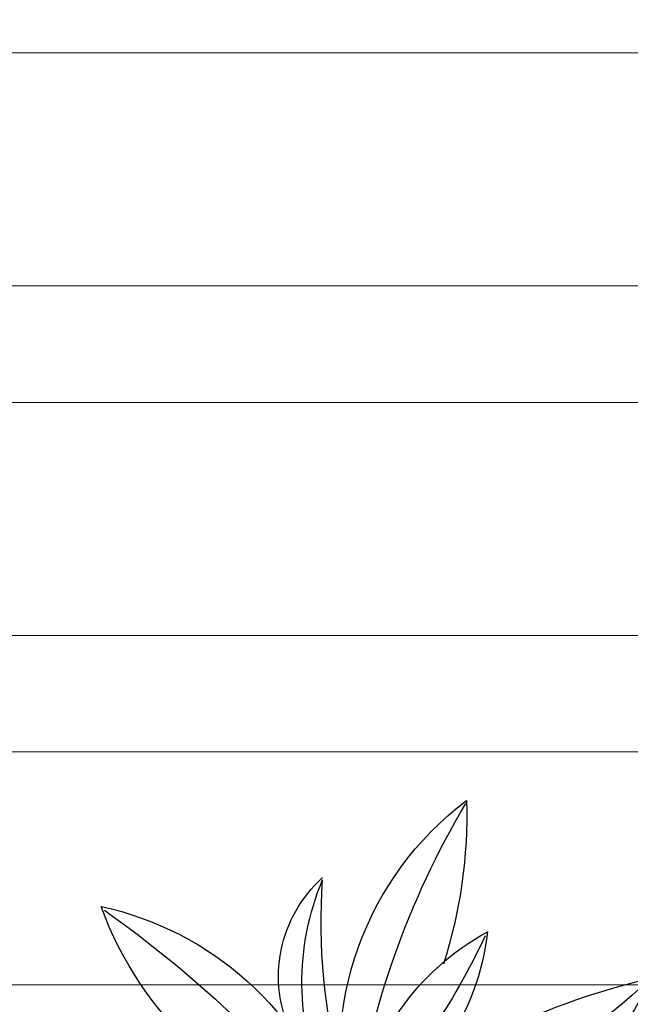
# Model space of a CAD drawing. Units: inches. Extents: x 351 to 1738, y -265 to 286.
# Tile 16 of 38: x 1176 to 1209, y -175 to -122. Entities that reach past the tile are written whole.
import ezdxf

# ---------------------------------------------------------------- set-up
doc = ezdxf.new("R2010")
doc.units = ezdxf.units.IN
doc.header["$MEASUREMENT"] = 0
doc.layers.add('A-ANNO-DIMS', color=2, linetype='Continuous', lineweight=18)
doc.layers.add('A-FLOR-PATT', color=9, linetype='Continuous', lineweight=9)
for name, color, linetype in [('CAY', 94, 'Continuous'), ('CHITIET', 144, 'Continuous'), ('netmanh', 9, 'Continuous'), ('VATDUNG', 9, 'Continuous')]:
    doc.layers.add(name, color=color, linetype=linetype)
doc.styles.get("Standard").update_dxf_attribs({"font": 'arial.ttf'})
doc.dimstyles.get("Standard").update_dxf_attribs({"dimtxt": 8, "dimasz": 5, "dimexe": 0.18, "dimexo": 0.0625, "dimgap": 0.09, "dimtad": 1, "dimtoh": 1, "dimzin": 0, "dimdsep": 46, "dimlunit": 4, "dimtxsty": 'Standard', "dimcen": 0, "dimclre": 256, "dimadec": 0, "dimazin": 0, "dimtfac": 1, "dimtofl": 0, "dimtmove": 0, "dimatfit": 3, "dimfxl": 1, "dimtolj": 1, "dimtzin": 0, "dimlwe": -1, "dimarcsym": 0})

# ---------------------------------------------------------------- blocks, each defined once
blk = doc.blocks.new('A$C5431134F')
at = {"layer": 'VATDUNG'}
for centre, radius, start, end in [((2160.8, 1662), 1245, 150.2411, 205.809), ((5177, 1582.5), 4150.3, 170.24, 186.1148), ((-65.9, 1738.8), 1267.2, 354.3326, 25.2804), ((193.1, 3473.3), 2507.8, 289.6318, 316.9416), ((2357.8, 162.2), 1629.1, 101.2486, 143.9899), ((1000.7, 2213.1), 1133.8, 274.4073, 336.4431), ((1532.8, 1250.1), 499, 101.4267, 190.9877), ((1828.1, 1082.8), 773.2, 121.9055, 175.1859), ((3715.1, 660.2), 2523.5, 154.6853, 162.4501), ((-246.7, 51.1), 1647.5, 39.15, 81.389), ((1000.7, 2213.1), 1133.8, 208.0484, 264.6491), ((1859.5, 3770.4), 2797.6, 228.5745, 252.3842), ((1101.5, 1552.5), 361.2, 169.1166, 218.9556), ((667.9, 1279.8), 349.9, 42.8374, 76.9786), ((-929.9, 388.9), 2082.1, 20.5138, 36.0242), ((1386.4, 1856.4), 738.5, 261.6389, 315.6255), ((-169.9, 6392.7), 5465.7, 286.3355, 292.415), ((1571.2, 1428.8), 356.3, 257.3557, 344.3532), ((624.5, 223.6), 940.4, 92.4374, 115.2956), ((-65.9, 1738.8), 1267.2, 330.7697, 331.9367), ((1294.4, -49.6), 1206.1, 104.1284, 160.1468), ((-2233.8, 3749.8), 4146.2, 305.4464, 320.7382), ((2052.7, 864.5), 1083.3, 166.3603, 232.9474), ((1250.8, 281.5), 836.9, 19.4342, 107.4357), ((625, 349.3), 851.8, 6.5073, 62.3609), ((-70, 1420), 1084.7, 282.2423, 341.7321), ((546.4, 1826.6), 819.5, 246.7315, 287.3971), ((248.9, 8461.8), 7388, 269.91003, 274.50199), ((3885.3, 1488.7), 2894, 188.0959, 210.7226), ((1889.6, 1210.8), 871.9, 188.5552, 241.3289), ((-527.8, -458.7), 2192.5, 24.7599, 44.6473), ((2594.9, 3037.7), 2500, 231.5416, 257.1764), ((754.1, -691.9), 1814.1, 46.1483, 80.3711), ((1738.9, 617.5), 897.6, 155.9893, 202.84), ((2946.5, 414), 2039.9, 165.0604, 184.0737), ((1214.1, 597.8), 452.1, 154.5276, 228.0163), ((-246.7, 51.1), 1647.5, 358.2222, 17.8583)]:
    blk.add_arc(centre, radius, start, end, dxfattribs=at)
blk = doc.blocks.new('A$C5A8625A6')
at = {"layer": 'CHITIET', "ltscale": 50, "xscale": -0.49, "yscale": 0.49, "zscale": 0.49, "rotation": 180}
blk.add_blockref('A$C5431134F', (0, 1120.2), dxfattribs=at)
blk = doc.blocks.new('A$C18571848')
at = {"layer": 'netmanh', "xscale": 0.5393606399999998, "yscale": 0.5393606399999998, "zscale": 0.5393606399999998}
blk.add_blockref('A$C5A8625A6', (0, 0), dxfattribs=at)
blk = doc.blocks.new('*D36')
at = {"layer": 'A-ANNO-DIMS', "transparency": 16777216}
for p, q in [((1073.569, -199.341), (1073.569, -204.202)), ((1105.198, -199.341), (1105.198, -204.202))]:
    blk.add_line(p, q, dxfattribs=at)
at = {"layer": 'A-ANNO-DIMS', "color": 0, "lineweight": -2, "transparency": 16777216}
for p, q in [((1078.569, -204.022), (1100.198, -204.022)), ((1105.198, -204.022), (1227.071, -204.022))]:
    blk.add_line(p, q, dxfattribs=at)
at = {"layer": 'A-ANNO-DIMS', "color": 0, "transparency": 16777216}
for points in [[(1078.569, -203.189), (1078.569, -204.856), (1073.569, -204.022)], [(1100.198, -203.189), (1100.198, -204.856), (1105.198, -204.022)]]:
    blk.add_solid(points, dxfattribs=at)
at = {"layer": 'Defpoints', "color": 0, "transparency": 16777216}
for p in [(1073.569, -199.278), (1105.198, -199.278), (1105.198, -204.022)]:
    blk.add_point(p, dxfattribs=at)
at = {"layer": 'A-ANNO-DIMS', "color": 0, "transparency": 16777216, "insert": (1168.634, -199.796), "char_height": 8, "attachment_point": 5}
blk.add_mtext('\\A1;PLANT A 2\'-7 1/2" TYP.', dxfattribs=at)

msp = doc.modelspace()

# ---------------------------------------------------------------- hatches: boundary and pattern name
at = {"layer": 'A-FLOR-PATT', "transparency": 33554559}
h = msp.add_hatch(dxfattribs=at)
h.set_pattern_fill('ANSI37', color=256, scale=200, angle=135)
h.set_pattern_definition([(180, (1112.704, -164.037), (-2e-15, -25), []), (270, (1112.704, -164.037), (25, -5e-15), [])])
h.paths.add_polyline_path([(1380.064, 73.463), (1380.132, 148.463), (1338.064, 148.463), (1290.704, 148.463), (1290.704, 88.463), (1248.704, 88.463), (1248.704, -2.009), (1244.704, -2.009), (1244.704, 142.457), (1160.704, 142.457), (1160.704, 158.963), (1160.704, 170.137), (1160.704, 206.137), (1160.704, 228.963), (1112.704, 228.963), (1112.704, 209.963), (1112.704, 168.963), (1124.704, 168.963), (1124.704, 162.963), (1112.704, 162.963), (1112.704, 64.463), (1112.704, 60.463), (1112.704, 0.463), (1112.704, -48.026), (1146.804, -47.981), (1146.804, -35.691), (1207.804, -35.691), (1207.804, -47.902), (1236.542, -47.864), (1236.544, -50.009), (1248.5, -50.009), (1248.506, -102.915), (1248.512, -150.915), (1248.514, -164.037), (1248.549, -164.037), (1273.017, -164.037), (1273.017, -128.799), (1355.24, -128.799), (1355.24, -164.037), (1384.204, -164.037), (1384.204, -57.037), (1380.064, -57.037), (1380.064, -48.037), (1392.064, -48.037), (1392.064, -53.037), (1406.549, -53.037), (1406.549, -57.037), (1401.204, -57.037), (1401.204, -147.037), (1468.204, -147.037), (1468.204, -138.5), (1472.204, -138.5), (1472.204, -102.5), (1468.204, -102.5), (1468.204, -57.037), (1442.549, -57.037), (1442.549, -53.037), (1463.049, -53.037), (1463.049, -40.747), (1524.049, -40.747), (1524.049, -48.037), (1536.064, -48.037), (1536.064, -53.037), (1557.704, -53.037), (1557.704, 204.963), (1384.204, 204.963), (1384.204, 73.463), (1392.064, 73.463), (1392.064, 64.463), (1384.204, 64.463), (1384.204, -3.5), (1380.204, -3.537), (1380.204, 64.463), (1380.064, 64.463)])
h.paths.add_polyline_path([(1510.714, 86.458, -0.103984), (1511.661, 85.595, 0.470438), (1510.158, 87.614, 0.0961)], flags=16)
h.paths.add_polyline_path([(1510.443, 100.266, 0.009798), (1504.693, 100.48, 0.02879), (1504.6, 99.767, -0.165331), (1505.519, 96.135, -0.143601)], flags=16)
h.paths.add_polyline_path([(1487.201, 85.595, -0.103984), (1488.148, 86.458, 0.0961), (1488.704, 87.614, 0.470438)], flags=0)
h.paths.add_polyline_path([(1495.052, 100.43), (1494.178, 100.43, -0.026463), (1494.262, 99.774, -0.144219)], flags=16)
h.paths.add_polyline_path([(1444.485, 86.458, -0.103984), (1445.433, 85.595, 0.470438), (1443.93, 87.614, 0.0961)], flags=16)
h.paths.add_polyline_path([(1420.972, 85.595, -0.103984), (1421.92, 86.458, 0.0961), (1422.475, 87.614, 0.470438)], flags=16)
h.paths.add_polyline_path([(1428.632, 100.335, 0.001054), (1427.971, 100.309, -0.021524), (1428.033, 99.774, -0.114301)], flags=16)
h.paths.add_polyline_path([(1419.906, 143.708, 0.024979), (1420.222, 157.526), (1421.573, 159.101), (1421.573, 175.369), (1391.393, 175.369), (1391.393, 200.519), (1542.294, 200.519), (1542.294, 175.369), (1512.028, 175.369, 0.019865), (1511.521, 153.838, 0.025134), (1512.758, 118.323, 0.020553), (1512.942, 115.253), (1419.834, 115.253, -0.000414), (1419.843, 124.798), (1413.059, 124.798), (1413.059, 84.437, -0.061853), (1415.831, 80.45, -0.093077), (1420.972, 85.595, -0.267537), (1422.371, 84.732, 0.08511), (1424.052, 84.616, -0.885393), (1424.033, 84.851, -1.125815), (1424.073, 84.366, -0.087987), (1422.371, 84.732, -0.267537), (1422.326, 83.089, -0.370542), (1420.972, 85.595, 0.093077), (1415.831, 80.45, -0.087414), (1417.914, 73.937), (1418.941, 73.937, 0.02725), (1418.913, 76.906, -0.115703), (1421.051, 73.937), (1445.354, 73.937, -0.115703), (1447.492, 76.906, 0.02725), (1447.464, 73.937), (1448.491, 73.937, -0.087414), (1450.574, 80.45, 0.093077), (1445.433, 85.595, -0.370542), (1444.079, 83.089, -0.267537), (1444.034, 84.732, -0.087987), (1442.332, 84.366, -1.125815), (1442.372, 84.851, -2.032736), (1442.364, 84.368, 0.086378), (1444.034, 84.732, -0.267537), (1445.433, 85.595, -0.093077), (1450.574, 80.45, -0.257732), (1466.483, 90.927, -0.47867), (1468.832, 91.907, -0.47867), (1471.18, 90.927, -0.26264), (1483.053, 81.78, -0.071866), (1487.201, 85.595, -0.267537), (1488.6, 84.732, 0.08511), (1490.28, 84.616, -0.885393), (1490.262, 84.851, -1.125815), (1490.301, 84.366, -0.087987), (1488.6, 84.732, -0.267537), (1488.554, 83.089, -0.370542), (1487.201, 85.595, 0.071866), (1483.053, 81.78, -0.132065), (1484.143, 73.937), (1485.169, 73.937, 0.02725), (1485.142, 76.906, -0.115703), (1487.28, 73.937), (1511.582, 73.937, -0.115703), (1513.72, 76.906, 0.02725), (1513.693, 73.937), (1514.719, 73.937, -0.087414), (1516.802, 80.45, 0.093077), (1511.661, 85.595, -0.370542), (1510.308, 83.089, -0.267537), (1510.262, 84.732, -0.087987), (1508.561, 84.366, -1.125815), (1508.601, 84.851, -2.032736), (1508.592, 84.368, 0.086378), (1510.262, 84.732, -0.267537), (1511.661, 85.595, -0.093077), (1516.802, 80.45, -0.061853), (1519.575, 84.437), (1519.575, 73.937), (1413.059, 73.937), (1413.059, 124.798), (1419.843, 124.798, -0.000821)], flags=16)
h.paths.add_polyline_path([(1220.149, 54.133, -0.103984), (1220.869, 53.476, 0.470438), (1219.727, 55.011, 0.0961)], flags=16)
h.paths.add_polyline_path([(1219.944, 64.626, 0.009798), (1215.574, 64.789, 0.02879), (1215.503, 64.247, -0.165331), (1216.201, 61.487, -0.143601)], flags=16)
h.paths.add_polyline_path([(1209.779, 64.449, 0.097446), (1209.339, 64.751), (1208.247, 64.751, 0.12739), (1207.7, 64.326, 0.171586), (1206.95, 61.475, -0.158854), (1207.636, 59.45, 0.015898), (1207.795, 59.218, 0.061546), (1208.598, 59.616, 0.175416), (1208.638, 60.099, -0.284779), (1209.348, 62.472, 0.326216)], flags=16)
h.paths.add_polyline_path([(1169.818, 54.133, -0.103984), (1170.538, 53.476, 0.470438), (1169.396, 55.011, 0.0961)], flags=16)
h.paths.add_polyline_path([(1159.017, 62.472, 0.284764), (1158.307, 60.099, -0.175433), (1158.267, 59.616, 0.39293), (1159.448, 64.449, -0.32623)], flags=16)
h.paths.add_polyline_path([(1156.342, 58.239, -0.178321), (1154.011, 55.31, -0.174736), (1154.722, 55.233, -0.200802), (1156.27, 56.086, 0.12699), (1157.283, 58.991, -0.091205)], flags=16)
h.paths.add_polyline_path([(1156.624, 61.413, 0.157275), (1157.316, 64.247, 0.169622)], flags=16)
h.paths.add_polyline_path([(1152.67, 54.133, -0.0961), (1151.95, 53.476, 0.064076), (1154.465, 54.384, 0.199016)], flags=16)
h.paths.add_polyline_path([(1202.281, 53.476, -0.103984), (1203, 54.133, 0.0961), (1203.423, 55.011, 0.470438)], flags=0)
h.paths.add_polyline_path([(1151.139, 97.64, 0.024979), (1151.379, 108.141), (1152.406, 109.338), (1152.406, 121.701), (1129.47, 121.701), (1129.47, 140.814), (1244.149, 140.814), (1244.149, 121.701), (1221.148, 121.701, 0.019865), (1220.763, 105.338, 0.025134), (1221.703, 78.349, 0.020553), (1221.843, 76.016), (1151.078, 76.016, -0.128743), (1148.786, 65.037, 0.539352), (1150.327, 64.171, -0.027594), (1163.481, 64.751, 0.097695), (1163.04, 64.449, 0.326216), (1163.471, 62.472, -0.284777), (1164.181, 60.099, -0.194757), (1165.846, 61.443, -0.155402), (1165.172, 64.247, -0.166022), (1165.869, 61.475, -0.177014), (1167.852, 62.77, -0.448203), (1169.974, 60.807, -0.393499), (1167.679, 57.86, -0.895548), (1168.438, 54.524, -0.355767), (1166.218, 56.086, -0.066024), (1165.505, 57.539), (1165.251, 56.243, -0.371732), (1164.02, 59.758, -0.373614), (1163.04, 64.449, -0.097695), (1163.481, 64.751, 0.021354), (1153.294, 64.429, -0.134183), (1156.695, 61.368, 0.186873), (1154.636, 62.77, 0.448203), (1152.514, 60.807, 0.403726), (1154.905, 57.846, 0.711219), (1153.334, 55, 0.53154), (1151.95, 53.476, -0.267537), (1153.013, 52.821, 0.08511), (1154.29, 52.732, -0.885393), (1154.276, 52.911, -1.125815), (1154.306, 52.543, -0.087987), (1153.013, 52.821, -0.267537), (1152.978, 51.572, -0.370542), (1151.95, 53.476, 0.093077), (1148.043, 49.566, -0.087414), (1149.626, 44.617), (1150.406, 44.617, 0.02725), (1150.385, 46.873, -0.115703), (1152.01, 44.617), (1170.478, 44.617, -0.115703), (1172.103, 46.873, 0.02725), (1172.082, 44.617), (1172.862, 44.617, -0.087414), (1174.445, 49.566, 0.093077), (1170.538, 53.476, -0.370542), (1169.51, 51.572, -0.267537), (1169.475, 52.821, -0.087987), (1168.182, 52.543, -1.125815), (1168.212, 52.911, -2.032736), (1168.206, 52.544, 0.086378), (1169.475, 52.821, -0.267537), (1170.538, 53.476, -0.093077), (1174.445, 49.566, -0.257732), (1186.536, 57.528, -0.47867), (1188.321, 58.273, -0.47867), (1190.106, 57.528, -0.26264), (1199.128, 50.577, -0.071866), (1202.281, 53.476, -0.267537), (1203.344, 52.821, 0.08511), (1204.621, 52.732, -0.885393), (1204.607, 52.911, -1.125815), (1204.637, 52.543, -0.087987), (1203.344, 52.821, -0.267537), (1203.309, 51.572, -0.370542), (1202.281, 53.476, 0.071866), (1199.128, 50.577, -0.132065), (1199.957, 44.617), (1200.737, 44.617, 0.02725), (1200.716, 46.873, -0.115703), (1202.341, 44.617), (1220.809, 44.617, -0.115703), (1222.434, 46.873, 0.02725), (1222.413, 44.617), (1223.193, 44.617, -0.087414), (1224.776, 49.566, 0.093077), (1220.869, 53.476, -0.370542), (1219.841, 51.572, -0.267537), (1219.806, 52.821, -0.087987), (1218.513, 52.543, -1.125815), (1218.543, 52.911, -2.032736), (1218.537, 52.544, 0.086378), (1219.806, 52.821, -0.267537), (1220.869, 53.476, -0.093077), (1224.776, 49.566, -0.061853), (1226.883, 52.597), (1226.883, 44.617), (1145.936, 44.617), (1145.936, 83.269), (1151.091, 83.269, -0.000821)], flags=16)
h.paths.add_polyline_path([(1218.01, 57.86, -0.895548), (1218.769, 54.524, -0.355767), (1216.549, 56.086, -0.066024), (1215.836, 57.539), (1215.582, 56.243, -0.371732), (1214.351, 59.758, -0.373614), (1213.371, 64.449, 0.326216), (1213.802, 62.472, -0.284777), (1214.512, 60.099, -0.194757), (1216.177, 61.443, -0.179991), (1218.183, 62.77, -0.448203), (1220.305, 60.807, -0.393499)], flags=16)
h.paths.add_polyline_path([(1424.735, 91.363, -0.393499), (1421.715, 95.241, -0.448203), (1424.507, 97.824, -0.179991), (1427.147, 96.077, -0.194757), (1429.338, 94.309, -0.284777), (1430.272, 97.432, 0.326216), (1430.839, 100.034, -0.373614), (1429.55, 93.861, -0.371732), (1427.929, 89.235), (1427.596, 90.941, -0.066024), (1426.657, 89.029, -0.355767), (1423.736, 86.973, -0.895548)], flags=16)
h.paths.add_polyline_path([(1238.033, 131.257, -1), (1227.329, 131.257, -1)], flags=0)
h.paths.add_polyline_path([(1235.357, 131.257, -1), (1230.005, 131.257, -1)], flags=0)
h.paths.add_polyline_path([(1214.039, 54.243, 0.154382), (1214.38, 53.992, 0.358955), (1213.613, 54.016, 0.603948), (1214.379, 53.657, 0.371319), (1213.968, 52.872, 0.187994), (1214.312, 52.809, -0.592455), (1213.953, 52.967, -0.294279), (1214.083, 53.691, -1.300187), (1213.881, 54.134, -0.283762), (1214.469, 53.896, 1.15094)], flags=16)
h.paths.add_polyline_path([(1212.091, 56.286, -0.408434), (1211.337, 56.445, -0.036259), (1211.098, 56.848, -0.236098), (1211.59, 56.63, 0.035345), (1211.835, 56.543, -0.475241), (1212.091, 56.286, -0.475241), (1212.438, 56.182, 0.035345), (1212.631, 56.007, -0.236098), (1213.056, 55.676, -0.036259), (1212.588, 55.697, -0.408434)], flags=16)
h.paths.add_polyline_path([(1211.469, 50.297, 0.296043), (1210.47, 50.527, 0.310883), (1211.931, 50.148, 0.021255)], flags=16)
h.paths.add_polyline_path([(1213.739, 51.818, -0.036259), (1213.271, 51.838, -0.408434), (1212.774, 52.427, -0.094786), (1212.293, 50.703, 1.150474), (1212.911, 50.232, 0.166288), (1213.265, 50.68, -0.025254), (1212.603, 50.13, 1.087932), (1212.471, 49.407, 0.166288), (1213.02, 49.251, -0.016128), (1212.567, 49.563, -0.286859), (1212.217, 49.638, 0.022156), (1212.046, 50.055, -0.64613), (1212.185, 50.498, 0.088412), (1212.732, 52.077, -1.186037), (1213.121, 52.323, 0.035345), (1213.314, 52.148, -0.236098)], flags=16)
h.paths.add_polyline_path([(1212.094, 50.342, -0.048524), (1211.54, 49.605, -1.103834), (1211.397, 48.738, -0.785515), (1211.683, 48.254, -0.392043), (1210.948, 48.525, -0.392819), (1210.561, 47.995, -0.592455), (1210.201, 48.153, -0.294279), (1210.331, 48.877, -0.704172), (1210.316, 49.592, -0.679344), (1210.729, 50.112, 0.563676)], flags=16)
h.paths.add_polyline_path([(1211.274, 49.829, -0.139826), (1210.745, 49.859, -0.217879), (1210.948, 49.509, -0.498572)], flags=0)
h.paths.add_polyline_path([(1433.426, 81.49, -0.181571), (1434.245, 81.788, -0.008067), (1433.726, 82.205, 0.045578), (1432.755, 81.242, 0.179011)], flags=16)
h.paths.add_polyline_path([(1434.146, 81.009, -0.132442), (1433.645, 80.771, 0.259089), (1433.234, 80.471, -0.180211), (1433.392, 80.805, -0.16994), (1432.758, 81.109, 0.032652), (1433.273, 80.474, -0.493363), (1434.046, 80.146, -0.390497)], flags=16)
h.paths.add_polyline_path([(1434.83, 80.047, -0.947538), (1435.294, 79.576, -0.299128), (1434.625, 79.404, -0.270439), (1435.01, 78.591, -0.592455), (1434.537, 78.382, -0.392819), (1434.027, 79.08, -0.392043), (1433.06, 78.723, -0.352042), (1433.003, 79.197, -0.197216), (1433.75, 79.734, -0.71364), (1434.447, 79.939, -0.21479), (1434.819, 80.475, 0.408833), (1435.075, 80.803, -0.226152)], flags=16)
h.paths.add_polyline_path([(1432.67, 81.217, -0.454218), (1431.897, 79.923, -0.414411), (1431.301, 80.035, 0.016129), (1431.897, 80.445, 0.27957), (1432.073, 80.871, -0.289504), (1431.103, 81.321, -0.414411), (1430.978, 81.915, 0.01613), (1431.586, 81.521, 0.341293), (1432.125, 81.583, -0.813186)], flags=16)
h.paths.add_polyline_path([(1429.893, 86.381, -0.947538), (1430.358, 85.91, -0.173106), (1429.984, 85.712, -0.038817), (1431.625, 84.214, -0.0879), (1432.097, 88.549, -0.049768), (1431.254, 88.49, -0.236098), (1431.814, 88.925, 0.035345), (1432.067, 89.155, -0.475241), (1432.524, 89.291, -0.475241), (1432.86, 89.63, 0.035345), (1433.182, 89.744, -0.236098), (1433.83, 90.032, -0.036259), (1433.516, 89.502, -0.408434), (1432.524, 89.291, -0.312424), (1432.106, 88.58, 0.088559), (1431.625, 84.214, -0.408434), (1430.971, 83.439, -0.036259), (1430.355, 83.412, -0.236098), (1430.914, 83.847, 0.035345), (1431.168, 84.078, -0.475241), (1431.625, 84.214, 0.038817), (1429.984, 85.712, -0.321732), (1429.333, 86.048, -0.32743), (1429.883, 86.809, 0.408833), (1430.138, 87.138, -0.226152)], flags=16)
h.paths.add_polyline_path([(1211.206, 58.616, -0.999784), (1211.336, 59.323, -0.614994)], flags=16)
h.paths.add_polyline_path([(1210.288, 49.429, 0.154382), (1210.629, 49.178, 0.358955), (1209.861, 49.202, 0.603948), (1210.627, 48.843, -0.534825), (1210.806, 49.295, 0.748346)], flags=16)
h.paths.add_polyline_path([(1209.589, 51.828, -0.008791), (1209.775, 51.753, 0.112231), (1209.466, 52.019, 1.418851), (1209.014, 51.708, -0.458726), (1208.651, 51.073, -0.592455), (1208.291, 51.232, -0.294279), (1208.421, 51.955, -1.300187), (1208.219, 52.398, -0.226005), (1208.719, 52.257, -0.475519), (1209.158, 52.369, -1.455499), (1209.603, 52.664, 0.421305), (1209.191, 52.262, -0.591212), (1208.979, 51.796, 0.497399), (1209.773, 51.333, 0.649312)], flags=16)
h.paths.add_polyline_path([(1208.029, 52.041, 0.544667), (1208.832, 52.045, 0.220132)], flags=0)
h.paths.add_polyline_path([(1210.438, 51.425, -0.2042), (1210.277, 52.018, 0.270826), (1209.915, 52.897, 0.324115)], flags=0)
h.paths.add_polyline_path([(1209.668, 52.407, -0.60139), (1208.99, 52.221, -0.394916), (1208.248, 52.83, -0.836792), (1208.651, 53.017, -0.338488), (1209.039, 52.571, 0.194138), (1209.191, 52.262, 0.413995), (1209.712, 52.475, 0.51771), (1210.503, 51.416, 0.401922), (1209.493, 50.93, 0.206396), (1209.516, 50.165, -0.319463), (1210.417, 51.418, -0.466635)], flags=16)
h.paths.add_polyline_path([(1206.601, 56.086, -0.355767), (1204.381, 54.524, -0.921198), (1205.236, 57.846, 0.206569), (1207.614, 58.991, -0.12699)], flags=16)
h.paths.add_polyline_path([(1435.487, 82.816, 0.527765), (1436.615, 83.361, 0.50854), (1437.05, 82.433, 0.592455), (1437.524, 82.641, 0.331245), (1436.963, 83.548, 0.387863), (1437.808, 83.626, 0.592954), (1437.618, 84.176, 0.226016), (1436.961, 83.99, 0.318205), (1437.588, 84.854, 0.689374), (1437.05, 84.991, 0.335765), (1436.539, 84.41, -0.156993), (1436.404, 84.065, -0.434611), (1436.961, 83.99, -0.21479), (1437.333, 84.526, 0.408833), (1437.588, 84.854, -0.226152), (1437.343, 84.097, -0.947538), (1437.808, 83.626, -0.299128), (1437.139, 83.455, -0.270439), (1437.524, 82.641, -0.592455), (1437.05, 82.433, -0.392819), (1436.541, 83.13, -0.43966), (1435.475, 82.794, -0.174614), (1435.942, 82.244, -0.206396), (1435.912, 81.237, -0.270826), (1435.125, 82.208, 0.207976), (1434.686, 82.904, -0.196495)], flags=16)
h.paths.add_polyline_path([(1435.386, 84.832, 0.270811), (1434.91, 83.676, -0.204217), (1434.699, 82.895, 0.324115)], flags=0)
h.paths.add_polyline_path([(1435.68, 84.18, -0.217656), (1435.554, 83.304, -0.176705), (1436.236, 83.778, -0.373036)], flags=0)
h.paths.add_polyline_path([(1435.566, 100.034, 0.326216), (1436.133, 97.432, -0.284777), (1437.067, 94.309, -0.194757), (1439.258, 96.077, -0.155402), (1438.371, 99.767, -0.166022), (1439.289, 96.12, -0.177014), (1441.897, 97.824, -0.448203), (1444.69, 95.241, -0.393499), (1441.67, 91.363, -0.895548), (1442.669, 86.973, -0.355767), (1439.748, 89.029, -0.066024), (1438.809, 90.941), (1438.476, 89.235, -0.371732), (1436.855, 93.861, -0.373614)], flags=16)
h.paths.add_polyline_path([(1191.252, 49.507, -0.274022), (1190.658, 48.409, 0.267537), (1191.311, 47.344, 0.370542)], flags=0)
h.paths.add_polyline_path([(1190.301, 49.717, 0.199016), (1188.619, 49.04, 0.064076), (1191.252, 49.507, -0.0961)], flags=0)
h.paths.add_polyline_path([(1189.518, 47.857, 1.125815), (1189.676, 47.523, 2.044605)], flags=0)
h.paths.add_polyline_path([(1464.974, 80.372, 0.274022), (1465.756, 78.927, -0.083013)], flags=0)
h.paths.add_polyline_path([(1464.974, 80.372, 0.370542), (1464.897, 77.525, 0.576324)], flags=0)
h.paths.add_polyline_path([(1464.974, 80.372, -0.470438), (1467.284, 81.372, -0.0961), (1466.226, 80.648, -0.199016), (1468.439, 79.757, -0.064076)], flags=0)
h.paths.add_polyline_path([(1189.511, 56.43, -0.259467), (1188.321, 56.391, -0.259467), (1187.13, 56.43, 0.08511), (1188.193, 55.716, -0.885393), (1188.27, 55.878, -1.196013), (1188.355, 55.442, 0.101459)], flags=0)
h.paths.add_polyline_path([(1188.321, 57.596, 0.078072), (1187.678, 57.24, 0.01555), (1188.321, 57.136, 0.01555), (1188.964, 57.24, 0.078072)], flags=0)
h.paths.add_polyline_path([(1190.164, 55.365, -0.576324), (1190.106, 57.528, -0.198294), (1188.321, 58.319, -0.198294), (1186.536, 57.528, -0.576324), (1186.477, 55.365, -0.370542), (1186.536, 57.528, 0.198294), (1188.321, 58.319, 0.198294), (1190.106, 57.528, -0.370542)], flags=0)
h.paths.add_polyline_path([(1188.372, 55.878, 1.125814), (1188.529, 55.544, 2.044605)], flags=0)
h.paths.add_polyline_path([(1186.341, 49.717, -0.0961), (1185.389, 49.507, 0.064076), (1188.022, 49.04, 0.199016)], flags=0)
h.paths.add_polyline_path([(1185.389, 49.507, -0.267537), (1185.984, 48.409, 0.08511), (1187.046, 47.695, -0.885393), (1187.123, 47.857, -1.125815), (1186.966, 47.523, -0.087987), (1185.984, 48.409, -0.267537), (1185.331, 47.344, -0.370542)], flags=0)
h.paths.add_polyline_path([(1399.441, 187.944, -1), (1413.525, 187.944, -1)], flags=0)
h.paths.add_polyline_path([(1402.962, 187.944, -1), (1410.004, 187.944, -1)], flags=0)
h.paths.add_polyline_path([(1357.663, -72.245), (1377.272, -72.245), (1377.272, -91.854), (1357.663, -91.854)], flags=16)
h.paths.add_polyline_path([(1467.256, 78.201, -1.125815), (1467.049, 77.761, -2.044605)], flags=0)
h.paths.add_polyline_path([(1468.822, 88.714, 0.941125), (1469.106, 88.316, 1.137152), (1468.765, 88.755, 0.890986), (1468.99, 88.245, 0.094828), (1470.398, 89.481, -0.267537), (1471.18, 90.927, -0.028123), (1469.678, 90.547, -0.028774), (1469.948, 90.311, -0.020327), (1468.832, 90.41, -0.020327), (1467.716, 90.311, -0.028774), (1467.986, 90.547, -0.028123), (1466.483, 90.927, -0.267537), (1467.265, 89.481, 0.08511), (1468.663, 88.542, -1.202316)], flags=0)
h.paths.add_polyline_path([(1178.25, 124.523, -0.119929), (1165.65, 124.145, -0.107349), (1159.133, 124.446, -0.102891), (1159.132, 130.465, -0.074897), (1158.993, 137.956, 0.002027), (1167.844, 137.479, -0.07553), (1180.337, 137.666, -0.075861), (1186.502, 137.688, -0.14099), (1186.272, 130.046, -0.095481), (1186.729, 124.748, -0.10603)], flags=0)
h.paths.add_polyline_path([(1469.225, 79.757, -0.199016), (1471.437, 80.648, -0.0961), (1470.379, 81.372, -0.470438), (1472.689, 80.372, -0.370542), (1472.766, 77.525, -0.267537), (1471.907, 78.927, -0.087986), (1470.615, 77.761, -1.125849), (1470.408, 78.201, -2.032736), (1470.642, 77.778, 0.086378), (1471.907, 78.927, -0.267537), (1472.689, 80.372, -0.064076)], flags=0)
h.paths.add_polyline_path([(1430.423, 186.902, -0.074897), (1430.24, 196.758, 0.002027), (1441.887, 196.131, -0.07553), (1458.326, 196.377, -0.075861), (1466.438, 196.406, -0.14099), (1466.136, 186.35, -0.095481), (1466.737, 179.378, -0.10603), (1455.58, 179.082, -0.119929), (1439, 178.585, -0.107349), (1430.425, 178.981, -0.102891)], flags=0)
h.paths.add_polyline_path([(1162.258, 49.939, 0.335765), (1161.87, 49.497, -0.156994), (1161.767, 49.235, -0.434611), (1162.19, 49.178, -0.21479), (1162.473, 49.585, 1.529195)], flags=16)
h.paths.add_polyline_path([(1161.683, 49.021, 0.581518), (1161.268, 49.583, 0.592761)], flags=16)
h.paths.add_polyline_path([(1162.602, 48.058, 0.371319), (1162.192, 48.843, 0.434533), (1162.88, 48.962, 0.185081), (1162.197, 48.926, 1.121837)], flags=16)
h.paths.add_polyline_path([(1161.443, 48.941, -1.307104), (1161.495, 48.571, -0.217752), (1161.136, 48.254, 0.697303), (1161.871, 49.048, 0.121514)], flags=16)
h.paths.add_polyline_path([(1162.531, 49.429, -0.207084), (1162.05, 49.146, -0.99203)], flags=16)
h.paths.add_polyline_path([(1161.304, 49.578, -0.719667), (1161.513, 50.079, -0.130428), (1160.836, 50.168, 0.039593)], flags=0)
h.paths.add_polyline_path([(1162.036, 50.584, -0.008067), (1161.642, 50.9, 0.029367), (1161.35, 50.297, -0.205788)], flags=16)
h.paths.add_polyline_path([(1162.882, 51.392, -0.124733), (1162.763, 51.828, -0.101191), (1162.399, 51.438, -0.153425)], flags=0)
h.paths.add_polyline_path([(1164.235, 51.85, -0.309107), (1164.513, 51.136, -0.627125), (1163.781, 51.603, -0.685909), (1162.777, 51.219, -0.233285), (1163.303, 50.165, -0.270826), (1162.705, 50.903, 0.2042), (1162.381, 51.425, 0.204182), (1162.542, 52.018, -0.270841), (1162.903, 52.897, -0.127261), (1163.219, 52.529, -1.168681), (1163.781, 52.587, -0.329112), (1164.168, 53.017, -0.836792), (1164.571, 52.83, -0.193341), (1164.391, 52.338, -0.947538), (1164.744, 51.981, -0.299128)], flags=16)
h.paths.add_polyline_path([(1163.598, 51.937, -1.262956), (1163.236, 51.831, 0.012575), (1162.971, 51.721, 0.230657), (1163.151, 52.407, -0.164898), (1163.178, 52.661, -0.44932), (1163.628, 52.262, -0.721477), (1164.154, 52.088, -0.849998)], flags=0)
h.paths.add_polyline_path([(1161.613, 58.616, -0.980413), (1161.525, 59.049, -2.908935)], flags=16)
h.paths.add_polyline_path([(1160.252, 49.166, -0.414411), (1159.799, 49.251, 0.016129), (1160.252, 49.563, 0.27957), (1160.386, 49.887, -0.289504), (1159.649, 50.229, -0.414411), (1159.554, 50.68, 0.01613), (1160.015, 50.381, 0.617885), (1160.526, 50.703, -0.094786), (1160.045, 52.427, -0.140444), (1159.682, 52.042, -0.057856), (1159.3, 51.872, 0.544843), (1160.046, 52.419, -0.088122), (1160.404, 55.721, -0.049768), (1159.763, 55.676, -0.236098), (1160.188, 56.007, 0.035345), (1160.381, 56.182, -0.475241), (1160.728, 56.286, -0.475241), (1160.984, 56.543, 0.035345), (1161.229, 56.63, -0.236098), (1161.721, 56.848, -0.036259), (1161.482, 56.445, -0.408434), (1160.728, 56.286, -0.312424), (1160.411, 55.745, 0.088559), (1160.045, 52.427, 0.107081), (1160.634, 50.498, -0.494798), (1160.839, 50.149, -0.454218)], flags=16)
h.paths.add_polyline_path([(1160.666, 49.808, -2.076528), (1160.828, 50.172, 0.019586)], flags=0)
h.paths.add_polyline_path([(1158.439, 53.992, 0.154382), (1158.78, 54.243, 0.748346), (1158.262, 54.109, -0.338225), (1158.492, 53.839, -0.170816), (1159.124, 53.779, 0.495729), (1158.938, 54.134, 0.226016)], flags=16)
h.paths.add_polyline_path([(1160.045, 52.427, 0.038817), (1158.798, 53.565, -0.119818), (1158.574, 53.586, -0.309107), (1158.851, 52.872, -0.187994), (1158.506, 52.809, 0.592455), (1158.866, 52.967, 0.331245), (1158.44, 53.657, 0.201245), (1158.798, 53.565, -0.034023), (1159.901, 52.578, -0.044253), (1159.698, 52.323, -0.475241)], flags=16)
h.paths.add_polyline_path([(1336.926, -95.392), (1336.926, -117.945), (1291.82, -117.945), (1291.82, -95.392)], flags=16)
h.paths.add_polyline_path([(1357.535, -97.244), (1357.726, -96.697, 0.034844)], flags=16)
h.paths.add_polyline_path([(1376.693, -96.478), (1377.301, -96.5, 0.031497), (1375.907, -96.424), (1357.726, -96.424)], flags=16)
h.paths.add_polyline_path([(1379.403, -119.667, 0.026706), (1380.043, -119.439, -0.015299)], flags=16)
h.paths.add_polyline_path([(1357.726, -120.202), (1357.821, -120.202), (1357.821, -120.201)], flags=16)
h.paths.add_polyline_path([(1354.171, -104.592), (1354.469, -98.672, 0.011138)], flags=16)
h.paths.add_polyline_path([(1355.058, -119.136), (1354.578, -118.539, 0.143164)], flags=16)
h.paths.add_polyline_path([(1378.851, -96.821), (1378.85, -96.82), (1378.85, -96.82, -0.04968), (1380.055, -97.191), (1378.85, -96.82, 0.150054), (1375.135, -97.188), (1375.136, -119.44, -0.00997), (1374.747, -116.649), (1357.726, -116.649, 0.169385), (1357.535, -119.382), (1357.535, -119.382), (1357.535, -119.382, 0.034818), (1357.726, -119.928), (1357.726, -119.928), (1357.726, -119.929, -0.034877), (1357.535, -119.382), (1355.507, -119.382), (1355.317, -119.278), (1357.535, -119.382, -0.169394), (1357.726, -116.649, -0.039151), (1374.686, -116.113, -0.002015), (1374.625, -115.546, 0.115322), (1369.915, -115.474, 0.060921), (1369.922, -101.154, 0.115146), (1374.625, -101.079, -0.002016), (1374.686, -100.513, -0.039151), (1357.726, -99.977), (1374.747, -99.977, -0.009963), (1375.135, -97.188), (1375.135, -97.188, -0.150108)], flags=16)
h.paths.add_polyline_path([(1490.963, 91.363, -0.393499), (1487.944, 95.241, -0.448203), (1490.736, 97.824, -0.179991), (1493.376, 96.077, -0.194757), (1495.567, 94.309, -0.284777), (1496.501, 97.432, 0.326216), (1497.068, 100.034, -0.373614), (1495.778, 93.861, -0.371732), (1494.158, 89.235), (1493.824, 90.941, -0.066024), (1492.886, 89.029, -0.355767), (1489.964, 86.973, -0.895548)], flags=16)
h.paths.add_polyline_path([(1354.86, -97.658), (1355.316, -97.348, 0.101911)], flags=16)
h.paths.add_polyline_path([(1497.063, 83.327, 0.176724), (1496.37, 83.785, -0.405139), (1496.016, 83.384, 0.497399), (1497.06, 82.774, 0.649312), (1496.818, 83.426, -0.008791)], flags=16)
h.paths.add_polyline_path([(1496.339, 83.783, 0.592761), (1496.886, 84.522, 0.581518)], flags=16)
h.paths.add_polyline_path([(1495.11, 82.641, 0.592455), (1495.583, 82.433, 0.676915), (1495.805, 83.59, 0.375669)], flags=16)
h.paths.add_polyline_path([(1495.015, 84.176, -0.145057), (1495.301, 84.526, -0.408833), (1495.045, 84.854, 0.220629), (1495.381, 84.152, -0.199594), (1495.851, 83.764, -0.524017), (1494.826, 83.626, -0.592998)], flags=16)
h.paths.add_polyline_path([(1501.655, 81.915, -0.016129), (1501.048, 81.521, -0.392719), (1500.462, 81.37, -0.21067), (1500.607, 81.142, 0.306699)], flags=16)
h.paths.add_polyline_path([(1500.11, 89.291, -0.408434), (1499.118, 89.502, -0.036259), (1498.803, 90.032, -0.236098), (1499.451, 89.744, 0.035345), (1499.774, 89.63, -0.475241), (1500.11, 89.291, -0.475241), (1500.567, 89.155, 0.035345), (1500.82, 88.925, -0.236098), (1501.379, 88.49, -0.036259), (1500.763, 88.516, -0.408434)], flags=16)
h.paths.add_polyline_path([(1498.908, 82.205, -0.051322), (1500.013, 81.134, -0.587931), (1500.234, 81.676, 0.107081), (1501.009, 84.214, -0.03529)], flags=16)
h.paths.add_polyline_path([(1496.93, 83.875, -0.206396), (1497.247, 84.832, -0.270826), (1497.724, 83.676, 0.207976), (1497.944, 82.884, -0.381455)], flags=16)
h.paths.add_polyline_path([(1496.721, 81.237, 0.270812), (1497.509, 82.208, -0.204216), (1497.935, 82.895, 0.324115)], flags=16)
h.paths.add_polyline_path([(1497.529, 80.125, -0.145057), (1497.814, 80.475, -0.703182), (1498.282, 81.178, -0.122925), (1497.977, 81.714, -0.270837), (1499.207, 81.49, 0.207964), (1499.993, 81.248, -0.265145), (1499.278, 80.472, 0.381901), (1498.808, 79.947, -0.305905), (1498.848, 79.519, 0.499482), (1498.574, 79.217, -0.458726), (1498.097, 78.382, -0.592455), (1497.624, 78.591, -0.270439), (1498.009, 79.404, -0.299116), (1497.34, 79.576, -0.593016)], flags=16)
h.paths.add_polyline_path([(1500.736, 79.923, 0.414411), (1501.333, 80.035, -0.321648), (1500.192, 80.765, 0.019886), (1499.976, 81.251, 0.465331)], flags=16)
h.paths.add_polyline_path([(1501.009, 84.214, -0.038817), (1502.649, 85.712, -0.173095), (1502.276, 85.91, -0.593016), (1502.465, 86.46, -0.145057), (1502.751, 86.809, -0.408833), (1502.495, 87.138, 0.220629), (1502.831, 86.436, -0.199594), (1503.301, 86.048, -0.321732), (1502.649, 85.712, 0.038817), (1501.009, 84.214, 0.122449), (1501.412, 83.755, 0.475491), (1501.335, 84.226, 0.055822), (1501.719, 83.847, -0.236098), (1502.278, 83.412, -0.036259), (1501.663, 83.439, -0.408434)], flags=16)
h.paths.add_polyline_path([(1501.794, 100.034, 0.326216), (1502.362, 97.432, -0.284777), (1503.295, 94.309, -0.194757), (1505.486, 96.077, -0.179991), (1508.126, 97.824, -0.448203), (1510.918, 95.241, -0.393499), (1507.899, 91.363, -0.895548), (1508.898, 86.973, -0.355767), (1505.976, 89.029, -0.066024), (1505.038, 90.941), (1504.704, 89.235, -0.371732), (1503.084, 93.861, -0.373614)], flags=16)
h.paths.add_polyline_path([(1146.29, 131.257, -1), (1135.587, 131.257, -1)], flags=0)
h.paths.add_polyline_path([(1143.614, 131.257, -1), (1138.262, 131.257, -1)], flags=0)
h.paths.add_polyline_path([(1524.064, 73.463), (1536.064, 73.463), (1536.064, 64.463), (1524.064, 64.463)], flags=16)
h.paths.add_polyline_path([(1520.162, 187.944, -1), (1534.246, 187.944, -1)], flags=0)
h.paths.add_polyline_path([(1530.725, 187.944), (1527.204, 187.944), (1527.204, 184.423, 0.414214)], flags=0)
h.paths.add_polyline_path([(1278.415, -91.154), (1331.067, -91.154), (1331.067, -80.583), (1278.415, -80.583)], flags=24)
h.paths.add_polyline_path([(1266.655, -79.354), (1354.738, -79.354), (1354.738, -67.817), (1266.655, -67.817)], flags=24)
h.paths.add_polyline_path([(1115.482, 206.184), (1155.098, 206.184), (1155.098, 217.714), (1115.482, 217.714)], flags=24)
h.paths.add_polyline_path([(1161.771, 8.501), (1222.466, 8.501), (1222.466, 19.079), (1161.771, 19.079)], flags=24)
h.paths.add_polyline_path([(1164.656, 18.795), (1210.615, 18.795), (1210.615, 30.324), (1164.656, 30.324)], flags=24)
h.paths.add_polyline_path([(1368.147, -32.882), (1379.362, -32.882), (1379.362, -21.733), (1368.147, -21.733)], flags=24)
h.paths.add_polyline_path([(1244.842, -31.012), (1256.057, -31.012), (1256.057, -19.863), (1244.842, -19.863)], flags=24)
h.paths.add_polyline_path([(1114.589, 195.739), (1156.517, 195.739), (1156.517, 206.31), (1114.589, 206.31)], flags=24)
h.paths.add_polyline_path([(1436.398, 37.632), (1505.131, 37.632), (1505.131, 48.203), (1436.398, 48.203)], flags=24)
h.paths.add_polyline_path([(1435.991, 47.919), (1507.906, 47.919), (1507.906, 59.456), (1435.991, 59.456)], flags=24)
h.paths.add_polyline_path([(1415.107, -124.896), (1457.038, -124.896), (1457.038, -114.318), (1415.107, -114.318)], flags=24)
h.paths.add_polyline_path([(1417.992, -114.602), (1457.609, -114.602), (1457.609, -103.073), (1417.992, -103.073)], flags=24)
h = msp.add_hatch(dxfattribs=at)
h.set_pattern_fill('ANSI32', color=256, scale=50, angle=135)
h.set_pattern_definition([(180, (1038.704, -199.037), (-2e-15, -18.75), []), (180, (1032.454, -192.787), (-2e-15, -18.75), [])])
h.paths.add_polyline_path([(1248.506, -102.915), (1236.559, -102.916), (1236.553, -56.864), (1112.704, -57.026), (1112.704, -57.037), (1103.704, -57.037), (1103.704, -45.037), (1103.704, 98.963), (1076.434, 98.963), (1076.549, -81.037), (1071.549, -81.037), (1043.704, -81.037), (1038.704, -81.037), (1038.704, -161.037), (1043.704, -161.037), (1043.704, -173.037), (1038.704, -173.037), (1038.704, -199.037), (1562.704, -199.037), (1562.704, -173.037), (1236.549, -173.037), (1236.549, -164.037), (1236.693, -164.037), (1236.676, -150.916), (1248.512, -150.915)])
h.paths.add_polyline_path([(1236.133, -134.078), (1247.348, -134.078), (1247.348, -122.929), (1236.133, -122.929)], flags=24)
h.paths.add_polyline_path([(1308.144, -185.548), (1321.66, -185.548), (1321.66, -174.4), (1308.144, -174.4)], flags=24)
h.paths.add_polyline_path([(1121.632, -122.88), (1179.647, -122.88), (1179.647, -112.309), (1121.632, -112.309)], flags=24)
h.paths.add_polyline_path([(1124.515, -112.593), (1177.986, -112.593), (1177.986, -101.056), (1124.515, -101.056)], flags=24)
h.paths.add_polyline_path([(1091.374, 23.58), (1104.89, 23.58), (1104.89, 34.728), (1091.374, 34.728)], flags=24)

# ---------------------------------------------------------------- block references
at = {"layer": 'CAY', "xscale": 0.0597507335965459, "yscale": 0.0597507335965459, "zscale": 0.0597507335965459}
msp.add_blockref('A$C18571848', (1177.835, -200.235), dxfattribs=at)

# ---------------------------------------------------------------- dimensions: what is measured, and where the dimension line sits
at = {"layer": 'A-ANNO-DIMS'}
dim = msp.add_linear_dim(base=(1105.198, -204.022), p1=(1073.569, -199.278), p2=(1105.198, -199.278), text='PLANT A <> TYP.', dimstyle='Standard', override={"dimdec": 1, "dimlfac": 1, "dimrnd": 0, "dimzin": 1, "dimdsep": 46, "dimlunit": 4, "dimfrac": 2}, dxfattribs=at)
dim.commit()
dim.dimension.update_dxf_attribs({"geometry": '*D36', "text_midpoint": (1168.634, -199.796)})

doc.saveas('drawing.dxf')
